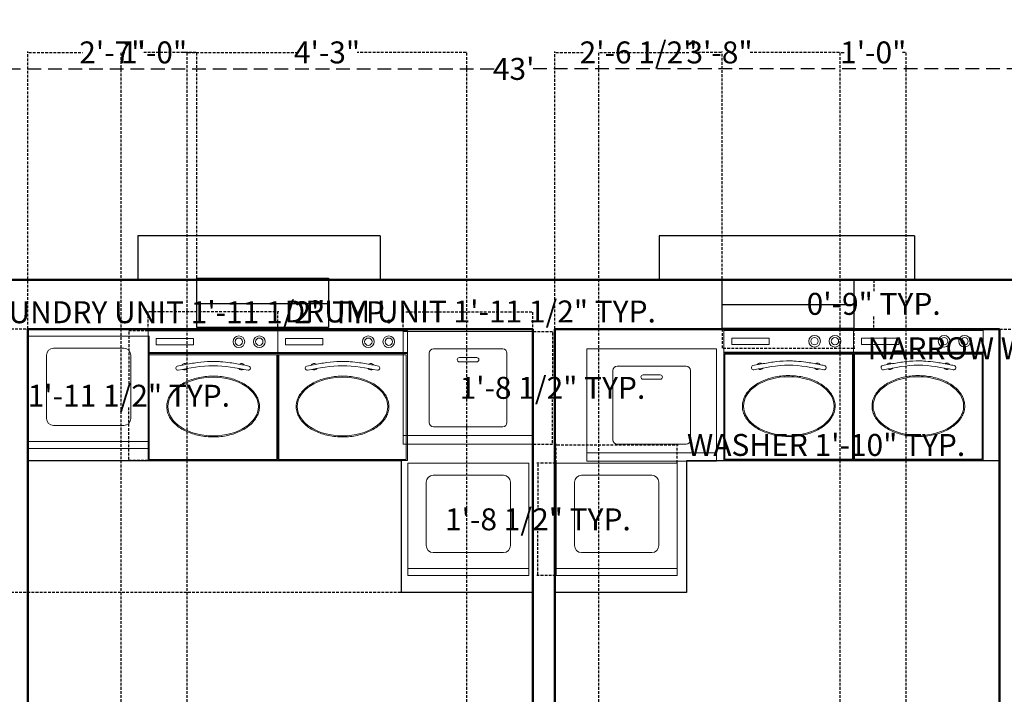
# Model space of a CAD drawing. Units: inches. Extents: x 513 to 1142, y 396 to 927.
# Tile 25 of 31: x 743 to 922, y 804 to 927. Entities that reach past the tile are written whole.
import ezdxf

# ---------------------------------------------------------------- set-up
doc = ezdxf.new("R2010")
doc.units = ezdxf.units.IN
doc.header["$MEASUREMENT"] = 0
doc.linetypes.add('DASHED', pattern=[0.75, 0.5, -0.25])
for name, color, linetype, lineweight in [('A-ANNO-DIMS', 2, 'DASHED', 18), ('A-EQPM', 92, 'Continuous', 18), ('A-FLOR-CASE', 7, 'Continuous', 25), ('A-WALL', 7, 'Continuous', 50), ('windows', 172, 'Continuous', 25)]:
    doc.layers.add(name, color=color, linetype=linetype, lineweight=lineweight)
doc.styles.get("Standard").update_dxf_attribs({"font": 'arial.ttf'})
doc.dimstyles.get("Standard").update_dxf_attribs({"dimtxt": 4, "dimasz": 0.18, "dimexe": 0.18, "dimexo": 0.0625, "dimgap": 0.09, "dimtad": 0, "dimtih": 1, "dimtoh": 1, "dimdec": 0, "dimrnd": 6, "dimzin": 0, "dimdsep": 46, "dimlunit": 3, "dimtxsty": 'Standard', "dimcen": 0.09, "dimadec": 0, "dimazin": 0, "dimtfac": 1, "dimtdec": 0, "dimtofl": 0, "dimtmove": 0, "dimatfit": 3, "dimfxl": 1, "dimtolj": 1, "dimtzin": 0, "dimarcsym": 0})

# ---------------------------------------------------------------- blocks, each defined once
blk = doc.blocks.new('A$C7E884C79')
for p, q in [((0, 0), (0, 600)), ((0, 600), (0, 0)), ((0, 600), (600, 600)), ((600, 600), (600, 0)), ((600, 0), (600, 600)), ((600, 600), (600, 450)), ((600, 600), (600, 500)), ((600, 500), (0, 500)), ((600, 495), (0, 495)), ((600, 500), (600, 0)), ((0, 0), (600, 0))]:
    blk.add_line(p, q)
for points in [[(36.4, 564.7), (208.9, 564.7), (208.9, 535.3), (36.4, 535.3)], [(5, 490), (595, 490), (595, 5), (5, 5)]]:
    blk.add_lwpolyline(points, close=True)
for centre, radius in [((419.3, 550), 27), ((419.3, 550), 17), ((513.9, 550), 27), ((513.9, 550), 17)]:
    blk.add_circle(centre, radius)
for centre, radius, start, end in [((137.2, 428), 10, 107.9829, 276.9581), ((168.5, 434.2), 15, 50.7888, 150.367), ((168.5, 434.2), 15, 234.0165, 327.1412), ((431.5, 434.2), 15, 212.8588, 305.9835), ((431.5, 434.2), 15, 29.633, 129.2112), ((462.8, 428), 10, 263.0419, 72.0171)]:
    blk.add_arc(centre, radius, start, end)
blk.add_ellipse((300, 250), major_axis=(-209.5, 0), ratio=0.648352)
for points, knots in [([(134.1, 437.5), (144.6, 439.5), (155.1, 441.6), (186, 447.3), (206.5, 450.9), (247.9, 456.4), (268.7, 458.3), (293.5, 458.9), (297.3, 458.9), (304.8, 458.9), (308.5, 458.8), (319.7, 458.5), (327.1, 458.1), (349.4, 456.5), (364.1, 454.9), (399.8, 449.9), (420.6, 446.2), (449.5, 440.7), (457.7, 439.1), (465.9, 437.5)], [0, 0, 0, 0, 31.638865, 31.638865, 92.600143, 92.600143, 153.561421, 153.561421, 164.367647, 164.367647, 175.173874, 175.173874, 196.786327, 196.786327, 240.011233, 240.011233, 302.099201, 302.099201, 326.773065, 326.773065, 326.773065, 326.773065]), ([(85.5, 250), (85.5, 244.8), (85.9, 239.6), (88, 226.9), (90.2, 219.4), (96.4, 204.8), (100.4, 197.7), (109.9, 184.1), (115.6, 177.5), (128.3, 165.1), (135.4, 159.2), (150.9, 148.3), (159.3, 143.3), (177.1, 134.2), (186.6, 130.1), (206.5, 123), (216.8, 119.9), (238.1, 114.9), (249, 113), (271.2, 110.2), (282.5, 109.4), (305, 109), (316.4, 109.4), (338.8, 111.3), (349.8, 112.8), (371.5, 117), (382.1, 119.6), (402.5, 126), (412.3, 129.7), (431, 138.1), (439.8, 142.8), (456.2, 153), (463.8, 158.6), (477.6, 170.5), (483.8, 176.8), (494.6, 190.1), (499.2, 197), (506.7, 211.3), (509.5, 218.7), (513.4, 233.6), (514.4, 241.3), (514.6, 256.5), (513.8, 264.1), (510.2, 279.1), (507.6, 286.6), (500.4, 300.9), (496, 307.9), (485.5, 321.3), (479.5, 327.7), (466, 339.7), (458.5, 345.3), (442.4, 355.8), (433.6, 360.5), (415.2, 369.1), (405.5, 373), (385.2, 379.5), (374.7, 382.3), (353.1, 386.7), (342, 388.3), (319.7, 390.5), (308.4, 390.9), (285.8, 390.7), (274.5, 390.1), (252.3, 387.5), (241.3, 385.7), (219.9, 380.9), (209.5, 378), (189.5, 371), (179.9, 367.1), (161.8, 358.1), (153.3, 353.2), (137.6, 342.5), (130.3, 336.7), (117.3, 324.4), (111.6, 317.9), (101.6, 304.3), (97.5, 297.3), (91, 282.8), (88.6, 275.3), (86, 261.9), (85.5, 255.9), (85.5, 250)], [0, 0, 0, 0, 0.108301, 0.108301, 0.267534, 0.267534, 0.426768, 0.426768, 0.586002, 0.586002, 0.745235, 0.745235, 0.904469, 0.904469, 1.063703, 1.063703, 1.222936, 1.222936, 1.38217, 1.38217, 1.541404, 1.541404, 1.700637, 1.700637, 1.859871, 1.859871, 2.019105, 2.019105, 2.178339, 2.178339, 2.337572, 2.337572, 2.496806, 2.496806, 2.65604, 2.65604, 2.815273, 2.815273, 2.974507, 2.974507, 3.133741, 3.133741, 3.292974, 3.292974, 3.452208, 3.452208, 3.611442, 3.611442, 3.770676, 3.770676, 3.929909, 3.929909, 4.089143, 4.089143, 4.248377, 4.248377, 4.40761, 4.40761, 4.566844, 4.566844, 4.726078, 4.726078, 4.885311, 4.885311, 5.044545, 5.044545, 5.203779, 5.203779, 5.363012, 5.363012, 5.522246, 5.522246, 5.68148, 5.68148, 5.840714, 5.840714, 5.999947, 5.999947, 6.159181, 6.159181, 6.283185, 6.283185, 6.283185, 6.283185])]:
    blk.add_open_spline(points, degree=3, knots=knots)
blk.add_open_spline([(138, 417.8), (192, 428.4), (300, 449.4), (408, 428.4), (462, 417.8)], degree=3)
blk = doc.blocks.new('LAVAD-01')
for p, q in [((-0.3221, 0.3585), (-0.3221, -0.3915)), ((0.3279, 0.3585), (-0.3221, 0.3585)), ((-0.2721, 0.3585), (-0.2721, -0.3915)), ((0.3279, -0.3915), (0.3279, 0.3585)), ((-0.2221, 0.1835), (-0.2221, -0.2165)), ((0.2029, 0.2085), (-0.1971, 0.2085)), ((0.2279, -0.2165), (0.2279, 0.1835)), ((0.1529, 0.0335), (0.1529, -0.0665)), ((0.1654, 0.046), (0.1654, 0.046)), ((0.1779, -0.0665), (0.1779, 0.0335)), ((0.1654, -0.079), (0.1654, -0.079)), ((-0.1971, -0.2415), (0.2029, -0.2415)), ((-0.3221, -0.3915), (0.3279, -0.3915))]:
    blk.add_line(p, q)
for centre, radius, start, end in [((-0.1971, 0.1835), 0.025, 90, 180), ((0.2029, 0.1835), 0.025, 0, 90), ((0.1654, 0.0335), 0.0125, 90, 180), ((0.1654, 0.0335), 0.0125, 0, 90), ((0.1654, -0.0665), 0.0125, 180, 270), ((0.1654, -0.0665), 0.0125, 270, 360), ((-0.1971, -0.2165), 0.025, 180, 270), ((0.2029, -0.2165), 0.025, 270, 360)]:
    blk.add_arc(centre, radius, start, end)
blk = doc.blocks.new('LAVADORA')
for p, q in [((-0.35, 0.65), (-0.35, 0)), ((-0.35, 0.65), (0.35, 0.65)), ((0.35, 0.65), (0.35, 0)), ((-0.2031, 0.5795), (0.2031, 0.5795)), ((-0.2437, 0.5389), (-0.2437, 0.1732)), ((0.2437, 0.5389), (0.2437, 0.1732)), ((-0.2031, 0.1326), (0.2031, 0.1326)), ((-0.35, 0.0406), (0.35, 0.0406)), ((-0.35, 0), (0.35, 0))]:
    blk.add_line(p, q)
for centre, start, end in [((-0.2031, 0.5389), 90, 180), ((0.2031, 0.5389), 0, 90), ((-0.2031, 0.1732), 180, 270), ((0.2031, 0.1732), 270, 0)]:
    blk.add_arc(centre, 0.0406, start, end)
blk = doc.blocks.new('*D103')
at = {"layer": 'A-ANNO-DIMS', "color": 0, "lineweight": -2, "ltscale": 5, "transparency": 16777216}
for p, q in [((575, 879.22), (575, 917.74)), ((575.18, 917.56), (828.93, 917.56)), ((1089.82, 917.56), (836.06, 917.56)), ((1090, 879.22), (1090, 917.74))]:
    blk.add_line(p, q, dxfattribs=at)
at = {"layer": 'A-ANNO-DIMS', "color": 0, "ltscale": 5, "transparency": 16777216}
for points in [[(575.18, 917.59), (575.18, 917.53), (575, 917.56)], [(1089.82, 917.59), (1089.82, 917.53), (1090, 917.56)]]:
    blk.add_solid(points, dxfattribs=at)
at = {"layer": 'Defpoints', "color": 0, "ltscale": 5, "transparency": 16777216}
for p in [(1090, 917.56), (575, 879.16), (1090, 879.16)]:
    blk.add_point(p, dxfattribs=at)
at = {"layer": 'A-ANNO-DIMS', "color": 0, "ltscale": 5, "transparency": 16777216, "insert": (832.5, 917.56), "char_height": 4, "attachment_point": 5}
blk.add_mtext("\\A1;43'", dxfattribs=at)
blk = doc.blocks.new('WIN-24IN')
blk.add_line((0, 4.39), (24, 4.39))
blk.add_lwpolyline([(24, 0), (0, 0), (0, 9), (24, 9)], close=True)
blk = doc.blocks.new('*D111')
at = {"layer": 'A-ANNO-DIMS', "color": 0, "lineweight": -2, "transparency": 16777216}
for p, q in [((765.94, 869.89), (765.94, 873.55)), ((789.56, 869.89), (789.56, 873.55)), ((766.12, 873.37), (789.38, 873.37)), ((789.56, 873.37), (789.74, 873.37))]:
    blk.add_line(p, q, dxfattribs=at)
at = {"layer": 'A-ANNO-DIMS', "color": 0, "transparency": 16777216}
for points in [[(766.12, 873.4), (766.12, 873.34), (765.94, 873.37)], [(789.38, 873.4), (789.38, 873.34), (789.56, 873.37)]]:
    blk.add_solid(points, dxfattribs=at)
at = {"layer": 'Defpoints', "color": 0, "transparency": 16777216}
for p in [(789.56, 873.37), (765.94, 869.83), (789.56, 869.83)]:
    blk.add_point(p, dxfattribs=at)
at = {"layer": 'A-ANNO-DIMS', "color": 0, "transparency": 16777216, "insert": (824.59, 873.37), "char_height": 4, "attachment_point": 5}
blk.add_mtext('\\A1;DRUM UNIT 1\'-11 1/2" TYP.', dxfattribs=at)
blk = doc.blocks.new('*D112')
at = {"layer": 'A-ANNO-DIMS', "color": 0, "lineweight": -2, "transparency": 16777216}
for p, q in [((765.88, 869.83), (762.22, 869.83)), ((762.4, 869.65), (762.4, 860.18)), ((762.4, 846.39), (762.4, 855.86)), ((765.88, 846.21), (762.22, 846.21))]:
    blk.add_line(p, q, dxfattribs=at)
at = {"layer": 'A-ANNO-DIMS', "color": 0, "transparency": 16777216}
for points in [[(762.37, 869.65), (762.43, 869.65), (762.4, 869.83)], [(762.37, 846.39), (762.43, 846.39), (762.4, 846.21)]]:
    blk.add_solid(points, dxfattribs=at)
at = {"layer": 'Defpoints', "color": 0, "transparency": 16777216}
for p in [(762.4, 869.83), (765.94, 869.83), (765.94, 846.21)]:
    blk.add_point(p, dxfattribs=at)
at = {"layer": 'A-ANNO-DIMS', "color": 0, "transparency": 16777216, "insert": (762.4, 858.02), "char_height": 4, "attachment_point": 5}
blk.add_mtext('\\A1;1\'-11 1/2" TYP.', dxfattribs=at)
blk = doc.blocks.new('*D113')
at = {"layer": 'A-ANNO-DIMS', "color": 0, "lineweight": -2, "transparency": 16777216}
for p, q in [((840.22, 845.81), (840.22, 849.24)), ((840.4, 849.06), (862.09, 849.06)), ((862.27, 845.81), (862.27, 849.24)), ((862.27, 849.06), (862.45, 849.06))]:
    blk.add_line(p, q, dxfattribs=at)
at = {"layer": 'A-ANNO-DIMS', "color": 0, "transparency": 16777216}
for points in [[(840.4, 849.09), (840.4, 849.03), (840.22, 849.06)], [(862.09, 849.09), (862.09, 849.03), (862.27, 849.06)]]:
    blk.add_solid(points, dxfattribs=at)
at = {"layer": 'Defpoints', "color": 0, "transparency": 16777216}
for p in [(862.27, 849.06), (840.22, 845.75), (862.27, 845.75)]:
    blk.add_point(p, dxfattribs=at)
at = {"layer": 'A-ANNO-DIMS', "color": 0, "transparency": 16777216, "insert": (889.41, 849.06), "char_height": 4, "attachment_point": 5}
blk.add_mtext('\\A1;WASHER 1\'-10" TYP.', dxfattribs=at)
blk = doc.blocks.new('*D114')
at = {"layer": 'A-ANNO-DIMS', "color": 0, "lineweight": -2, "transparency": 16777216}
for p, q in [((840.16, 845.75), (836.74, 845.75)), ((836.92, 845.57), (836.92, 837.67)), ((836.92, 825.46), (836.92, 833.35)), ((840.16, 825.28), (836.74, 825.28))]:
    blk.add_line(p, q, dxfattribs=at)
at = {"layer": 'A-ANNO-DIMS', "color": 0, "transparency": 16777216}
for points in [[(836.89, 845.57), (836.95, 845.57), (836.92, 845.75)], [(836.89, 825.46), (836.95, 825.46), (836.92, 825.28)]]:
    blk.add_solid(points, dxfattribs=at)
at = {"layer": 'Defpoints', "color": 0, "transparency": 16777216}
for p in [(836.92, 845.75), (840.22, 845.75), (840.22, 825.28)]:
    blk.add_point(p, dxfattribs=at)
at = {"layer": 'A-ANNO-DIMS', "color": 0, "transparency": 16777216, "insert": (836.92, 835.51), "char_height": 4, "attachment_point": 5}
blk.add_mtext('\\A1;1\'-8 1/2" TYP.', dxfattribs=at)
blk = doc.blocks.new('*D115')
at = {"layer": 'A-ANNO-DIMS', "color": 0, "lineweight": -2, "transparency": 16777216}
for p, q in [((812.39, 873.24), (812.21, 873.24)), ((812.39, 869.76), (812.39, 873.42)), ((835.83, 873.24), (812.57, 873.24)), ((836.01, 869.76), (836.01, 873.42))]:
    blk.add_line(p, q, dxfattribs=at)
at = {"layer": 'A-ANNO-DIMS', "color": 0, "transparency": 16777216}
for points in [[(812.57, 873.27), (812.57, 873.21), (812.39, 873.24)], [(835.83, 873.27), (835.83, 873.21), (836.01, 873.24)]]:
    blk.add_solid(points, dxfattribs=at)
at = {"layer": 'Defpoints', "color": 0, "transparency": 16777216}
for p in [(812.39, 873.24), (812.39, 869.7), (836.01, 869.7)]:
    blk.add_point(p, dxfattribs=at)
at = {"layer": 'A-ANNO-DIMS', "color": 0, "transparency": 16777216, "insert": (772.38, 873.24), "char_height": 4, "attachment_point": 5}
blk.add_mtext('\\A1;LAUNDRY UNIT 1\'-11 1/2" TYP.', dxfattribs=at)
blk = doc.blocks.new('*D116')
at = {"layer": 'A-ANNO-DIMS', "color": 0, "lineweight": -2, "transparency": 16777216}
for p, q in [((836.08, 869.7), (839.74, 869.7)), ((839.56, 869.52), (839.56, 861.62)), ((839.56, 849.41), (839.56, 857.31)), ((836.08, 849.23), (839.74, 849.23))]:
    blk.add_line(p, q, dxfattribs=at)
at = {"layer": 'A-ANNO-DIMS', "color": 0, "transparency": 16777216}
for points in [[(839.53, 869.52), (839.59, 869.52), (839.56, 869.7)], [(839.53, 849.41), (839.59, 849.41), (839.56, 849.23)]]:
    blk.add_solid(points, dxfattribs=at)
at = {"layer": 'Defpoints', "color": 0, "transparency": 16777216}
for p in [(836.01, 869.7), (839.56, 869.7), (836.01, 849.23)]:
    blk.add_point(p, dxfattribs=at)
at = {"layer": 'A-ANNO-DIMS', "color": 0, "transparency": 16777216, "insert": (839.56, 859.46), "char_height": 4, "attachment_point": 5}
blk.add_mtext('\\A1;1\'-8 1/2" TYP.', dxfattribs=at)
blk = doc.blocks.new('*D129')
at = {"layer": 'A-ANNO-DIMS', "color": 0, "lineweight": -2, "transparency": 16777216}
for p, q in [((870.48, 870.2), (870.48, 866.48)), ((894.48, 870.2), (894.48, 866.48)), ((870.66, 866.66), (894.3, 866.66)), ((894.48, 866.66), (894.66, 866.66))]:
    blk.add_line(p, q, dxfattribs=at)
at = {"layer": 'A-ANNO-DIMS', "color": 0, "transparency": 16777216}
for points in [[(870.66, 866.69), (870.66, 866.63), (870.48, 866.66)], [(894.3, 866.69), (894.3, 866.63), (894.48, 866.66)]]:
    blk.add_solid(points, dxfattribs=at)
at = {"layer": 'Defpoints', "color": 0, "transparency": 16777216}
for p in [(870.48, 870.26), (894.48, 870.26), (894.48, 866.66)]:
    blk.add_point(p, dxfattribs=at)
at = {"layer": 'A-ANNO-DIMS', "color": 0, "transparency": 16777216, "insert": (933.38, 866.66), "char_height": 4, "attachment_point": 5}
blk.add_mtext('\\A1;NARROW WINDOW 2\'-0" TYP.', dxfattribs=at)
blk = doc.blocks.new('*D130')
at = {"layer": 'A-ANNO-DIMS', "color": 0, "lineweight": -2, "transparency": 16777216}
for p, q in [((894.54, 879.26), (898.26, 879.26)), ((898.08, 879.08), (898.08, 876.9)), ((898.08, 870.44), (898.08, 872.63)), ((894.54, 870.26), (898.26, 870.26))]:
    blk.add_line(p, q, dxfattribs=at)
at = {"layer": 'A-ANNO-DIMS', "color": 0, "transparency": 16777216}
for points in [[(898.05, 879.08), (898.11, 879.08), (898.08, 879.26)], [(898.05, 870.44), (898.11, 870.44), (898.08, 870.26)]]:
    blk.add_solid(points, dxfattribs=at)
at = {"layer": 'Defpoints', "color": 0, "transparency": 16777216}
for p in [(894.48, 879.26), (898.08, 879.26), (894.48, 870.26)]:
    blk.add_point(p, dxfattribs=at)
at = {"layer": 'A-ANNO-DIMS', "color": 0, "transparency": 16777216, "insert": (898.08, 874.76), "char_height": 4, "attachment_point": 5}
blk.add_mtext('\\A1;0\'-9" TYP.', dxfattribs=at)
blk = doc.blocks.new('*D148')
at = {"layer": 'A-ANNO-DIMS', "color": 0, "lineweight": -2, "transparency": 16777216}
for p, q in [((921.06, 870.16), (1131.58, 870.16)), ((1131.4, 869.98), (1131.4, 824.29)), ((1131.4, 774.34), (1131.4, 820.03)), ((897.06, 774.16), (1131.58, 774.16))]:
    blk.add_line(p, q, dxfattribs=at)
at = {"layer": 'A-ANNO-DIMS', "color": 0, "transparency": 16777216}
for points in [[(1131.37, 869.98), (1131.43, 869.98), (1131.4, 870.16)], [(1131.37, 774.34), (1131.43, 774.34), (1131.4, 774.16)]]:
    blk.add_solid(points, dxfattribs=at)
at = {"layer": 'Defpoints', "color": 0, "transparency": 16777216}
for p in [(921, 870.16), (1131.4, 870.16), (897, 774.16)]:
    blk.add_point(p, dxfattribs=at)
at = {"layer": 'A-ANNO-DIMS', "color": 0, "transparency": 16777216, "insert": (1131.4, 822.16), "char_height": 4, "attachment_point": 5}
blk.add_mtext('\\A1;8\'-0"', dxfattribs=at)
blk = doc.blocks.new('*D153')
at = {"layer": 'A-ANNO-DIMS', "color": 0, "lineweight": -2, "transparency": 16777216}
for p, q in [((744, 870.22), (744, 920.74)), ((744.18, 920.56), (753.95, 920.56)), ((774.61, 920.56), (764.83, 920.56)), ((774.79, 870.5), (774.79, 920.74))]:
    blk.add_line(p, q, dxfattribs=at)
at = {"layer": 'A-ANNO-DIMS', "color": 0, "transparency": 16777216}
for points in [[(744.18, 920.59), (744.18, 920.53), (744, 920.56)], [(774.61, 920.59), (774.61, 920.53), (774.79, 920.56)]]:
    blk.add_solid(points, dxfattribs=at)
at = {"layer": 'Defpoints', "color": 0, "transparency": 16777216}
for p in [(774.79, 920.56), (744, 870.16), (774.79, 870.44)]:
    blk.add_point(p, dxfattribs=at)
at = {"layer": 'A-ANNO-DIMS', "color": 0, "transparency": 16777216, "insert": (759.39, 920.56), "char_height": 4, "attachment_point": 5}
blk.add_mtext('\\A1;2\'-7"', dxfattribs=at)
blk = doc.blocks.new('*D154')
at = {"layer": 'A-ANNO-DIMS', "color": 0, "lineweight": -2, "transparency": 16777216}
for p, q in [((840, 870.22), (840, 920.74)), ((840.18, 920.56), (845.14, 920.56)), ((870.3, 920.56), (865.34, 920.56)), ((870.48, 870.33), (870.48, 920.74))]:
    blk.add_line(p, q, dxfattribs=at)
at = {"layer": 'A-ANNO-DIMS', "color": 0, "transparency": 16777216}
for points in [[(840.18, 920.59), (840.18, 920.53), (840, 920.56)], [(870.3, 920.59), (870.3, 920.53), (870.48, 920.56)]]:
    blk.add_solid(points, dxfattribs=at)
at = {"layer": 'Defpoints', "color": 0, "transparency": 16777216}
for p in [(870.48, 920.56), (840, 870.16), (870.48, 870.26)]:
    blk.add_point(p, dxfattribs=at)
at = {"layer": 'A-ANNO-DIMS', "color": 0, "transparency": 16777216, "insert": (855.24, 920.56), "char_height": 4, "attachment_point": 5}
blk.add_mtext('\\A1;2\'-6 1/2"', dxfattribs=at)
blk = doc.blocks.new('*D167')
at = {"layer": 'A-ANNO-DIMS', "color": 0, "lineweight": -2, "transparency": 16777216}
for p, q in [((761, 637.22), (761, 920.74)), ((761.18, 920.56), (761.78, 920.56)), ((772.82, 920.56), (772.21, 920.56)), ((773, 637.22), (773, 920.74))]:
    blk.add_line(p, q, dxfattribs=at)
at = {"layer": 'A-ANNO-DIMS', "color": 0, "transparency": 16777216}
for points in [[(761.18, 920.59), (761.18, 920.53), (761, 920.56)], [(772.82, 920.59), (772.82, 920.53), (773, 920.56)]]:
    blk.add_solid(points, dxfattribs=at)
at = {"layer": 'Defpoints', "color": 0, "transparency": 16777216}
for p in [(773, 920.56), (761, 637.16), (773, 637.16)]:
    blk.add_point(p, dxfattribs=at)
at = {"layer": 'A-ANNO-DIMS', "color": 0, "transparency": 16777216, "insert": (767, 920.56), "char_height": 4, "attachment_point": 5}
blk.add_mtext('\\A1;1\'-0"', dxfattribs=at)
blk = doc.blocks.new('*D168')
at = {"layer": 'A-ANNO-DIMS', "color": 0, "lineweight": -2, "transparency": 16777216}
for p, q in [((892, 637.22), (892, 920.74)), ((892.18, 920.56), (892.78, 920.56)), ((903.82, 920.56), (903.21, 920.56)), ((904, 637.22), (904, 920.74))]:
    blk.add_line(p, q, dxfattribs=at)
at = {"layer": 'A-ANNO-DIMS', "color": 0, "transparency": 16777216}
for points in [[(892.18, 920.59), (892.18, 920.53), (892, 920.56)], [(903.82, 920.59), (903.82, 920.53), (904, 920.56)]]:
    blk.add_solid(points, dxfattribs=at)
at = {"layer": 'Defpoints', "color": 0, "transparency": 16777216}
for p in [(904, 920.56), (892, 637.16), (904, 637.16)]:
    blk.add_point(p, dxfattribs=at)
at = {"layer": 'A-ANNO-DIMS', "color": 0, "transparency": 16777216, "insert": (898, 920.56), "char_height": 4, "attachment_point": 5}
blk.add_mtext('\\A1;1\'-0"', dxfattribs=at)
blk = doc.blocks.new('*D170')
at = {"layer": 'A-ANNO-DIMS', "color": 0, "lineweight": -2, "transparency": 16777216}
for p, q in [((835.93, 870.16), (533.42, 870.16)), ((533.6, 869.98), (533.6, 848.29)), ((533.6, 822.34), (533.6, 844.03)), ((835.93, 822.16), (533.42, 822.16))]:
    blk.add_line(p, q, dxfattribs=at)
at = {"layer": 'A-ANNO-DIMS', "color": 0, "transparency": 16777216}
for points in [[(533.57, 869.98), (533.63, 869.98), (533.6, 870.16)], [(533.57, 822.34), (533.63, 822.34), (533.6, 822.16)]]:
    blk.add_solid(points, dxfattribs=at)
at = {"layer": 'Defpoints', "color": 0, "transparency": 16777216}
for p in [(533.6, 870.16), (836, 870.16), (836, 822.16)]:
    blk.add_point(p, dxfattribs=at)
at = {"layer": 'A-ANNO-DIMS', "color": 0, "transparency": 16777216, "insert": (533.6, 846.16), "char_height": 4, "attachment_point": 5}
blk.add_mtext('\\A1;4\'-0"', dxfattribs=at)
blk = doc.blocks.new('*D175')
at = {"layer": 'A-ANNO-DIMS', "color": 0, "lineweight": -2, "transparency": 16777216}
for p, q in [((773, 637.22), (773, 920.74)), ((773.18, 920.56), (793.01, 920.56)), ((823.82, 920.56), (803.98, 920.56)), ((824, 637.22), (824, 920.74))]:
    blk.add_line(p, q, dxfattribs=at)
at = {"layer": 'A-ANNO-DIMS', "color": 0, "transparency": 16777216}
for points in [[(773.18, 920.59), (773.18, 920.53), (773, 920.56)], [(823.82, 920.59), (823.82, 920.53), (824, 920.56)]]:
    blk.add_solid(points, dxfattribs=at)
at = {"layer": 'Defpoints', "color": 0, "transparency": 16777216}
for p in [(824, 920.56), (773, 637.16), (824, 637.16)]:
    blk.add_point(p, dxfattribs=at)
at = {"layer": 'A-ANNO-DIMS', "color": 0, "transparency": 16777216, "insert": (798.5, 920.56), "char_height": 4, "attachment_point": 5}
blk.add_mtext('\\A1;4\'-3"', dxfattribs=at)
blk = doc.blocks.new('*D176')
at = {"layer": 'A-ANNO-DIMS', "color": 0, "lineweight": -2, "transparency": 16777216}
for p, q in [((848, 637.22), (848, 920.74)), ((848.18, 920.56), (864.59, 920.56)), ((891.82, 920.56), (875.4, 920.56)), ((892, 637.22), (892, 920.74))]:
    blk.add_line(p, q, dxfattribs=at)
at = {"layer": 'A-ANNO-DIMS', "color": 0, "transparency": 16777216}
for points in [[(848.18, 920.59), (848.18, 920.53), (848, 920.56)], [(891.82, 920.59), (891.82, 920.53), (892, 920.56)]]:
    blk.add_solid(points, dxfattribs=at)
at = {"layer": 'Defpoints', "color": 0, "transparency": 16777216}
for p in [(892, 920.56), (848, 637.16), (892, 637.16)]:
    blk.add_point(p, dxfattribs=at)
at = {"layer": 'A-ANNO-DIMS', "color": 0, "transparency": 16777216, "insert": (870, 920.56), "char_height": 4, "attachment_point": 5}
blk.add_mtext('\\A1;3\'-8"', dxfattribs=at)

msp = doc.modelspace()

# ---------------------------------------------------------------- linework, layer by layer
at = {"layer": 'A-FLOR-CASE'}
for p, q in [((812, 846.16), (744, 846.16)), ((812, 846.16), (812, 822.16)), ((921, 846.16), (864, 846.16)), ((864, 846.16), (864, 822.16)), ((836, 822.16), (812, 822.16)), ((864, 822.16), (840, 822.16))]:
    msp.add_line(p, q, dxfattribs=at)
at = {"layer": 'A-WALL'}
for p, q in [((1090, 879.16), (575, 879.16)), ((744, 870.16), (744, 710.16)), ((836, 870.16), (744, 870.16)), ((836, 870.16), (836, 774.16)), ((840, 870.16), (840, 774.16)), ((921, 870.16), (840, 870.16)), ((921, 710.16), (921, 870.16))]:
    msp.add_line(p, q, dxfattribs=at)
at = {"layer": 'windows'}
for p, q in [((764.02, 887.16), (764.02, 879.16)), ((808.21, 887.16), (764.02, 887.16)), ((808.21, 887.16), (808.21, 879.16)), ((859.02, 887.16), (859.02, 879.16)), ((905.5, 887.16), (859.02, 887.16)), ((905.5, 887.16), (905.5, 879.16))]:
    msp.add_line(p, q, dxfattribs=at)

# ---------------------------------------------------------------- block references
at = {"layer": 'A-EQPM'}
for name, p, xscale, yscale, zscale in [('A$C7E884C79', (870.8, 846.3), 0.0393700787401575, 0.0393700787401575, 0.0393700787401575), ('A$C7E884C79', (894.41, 846.3), 0.0393700787401575, 0.0393700787401575, 0.0393700787401575), ('LAVADORA', (755.08, 848.43), 31.49606299212599, 31.49606299212599, 31.49606299212599), ('A$C7E884C79', (765.94, 846.21), 0.0393700787401575, 0.0393700787401575, 0.0393700787401575), ('A$C7E884C79', (789.52, 846.21), 0.0393700787401575, 0.0393700787401575, 0.0393700787401575), ('LAVADORA', (824.25, 825.28), 31.49606299212599, 31.49606299212599, 31.49606299212599), ('LAVADORA', (851.25, 825.28), 31.49606299212599, 31.49606299212599, 31.49606299212599)]:
    msp.add_blockref(name, p, dxfattribs=dict(at, xscale=xscale, yscale=yscale, zscale=zscale))
at = {"layer": 'A-EQPM', "xscale": 31.49606299212599, "yscale": 31.49606299212599, "zscale": 31.49606299212599, "rotation": 90}
for p in [(823.68, 859.37), (857.12, 856.22)]:
    msp.add_blockref('LAVAD-01', p, dxfattribs=at)
at = {"layer": 'windows'}
for p in [(774.79, 870.44), (870.48, 870.26)]:
    msp.add_blockref('WIN-24IN', p, dxfattribs=at)

# ---------------------------------------------------------------- dimensions: what is measured, and where the dimension line sits
at = {"layer": 'A-ANNO-DIMS'}
for base, p1, p2, picture, middle in [((870.48, 920.56), (840, 870.16), (870.48, 870.26), '*D154', (855.24, 920.56)), ((774.79, 920.56), (744, 870.16), (774.79, 870.44), '*D153', (759.39, 920.56)), ((773, 920.56), (761, 637.16), (773, 637.16), '*D167', (767, 920.56)), ((824, 920.56), (773, 637.16), (824, 637.16), '*D175', (798.5, 920.56)), ((892, 920.56), (848, 637.16), (892, 637.16), '*D176', (870, 920.56)), ((904, 920.56), (892, 637.16), (904, 637.16), '*D168', (898, 920.56))]:
    dim = msp.add_linear_dim(base=base, p1=p1, p2=p2, dimstyle='Standard', override={"dimdec": 1, "dimlfac": 1, "dimrnd": 0, "dimzin": 1, "dimdsep": 46, "dimlunit": 4, "dimfrac": 2}, dxfattribs=at)
    dim.commit()
    dim.dimension.update_dxf_attribs({"geometry": picture, "text_midpoint": middle})
at = {"layer": 'A-ANNO-DIMS', "ltscale": 5}
dim = msp.add_linear_dim(base=(1090, 917.56), p1=(575, 879.16), p2=(1090, 879.16), dimstyle='Standard', override={"dimclrd": 0, "dimclre": 0, "dimclrt": 0}, dxfattribs=at)
dim.commit()
dim.dimension.update_dxf_attribs({"geometry": '*D103', "text_midpoint": (832.5, 917.56)})
at = {"layer": 'A-ANNO-DIMS'}
for base, p1, p2, angle, text, picture, middle in [((812.39, 873.24), (836.01, 869.7), (812.39, 869.7), 180, 'LAUNDRY UNIT <> TYP.', '*D115', (772.38, 873.24)), ((898.08, 879.26), (894.48, 870.26), (894.48, 879.26), 90, '<> TYP.', '*D130', (898.08, 874.76)), ((762.4, 869.83), (765.94, 846.21), (765.94, 869.83), 90, '<> TYP.', '*D112', (762.4, 858.02)), ((839.56, 869.7), (836.01, 849.23), (836.01, 869.7), 90, '<> TYP.', '*D116', (839.56, 859.46)), ((836.92, 845.75), (840.22, 825.28), (840.22, 845.75), 90, '<> TYP.', '*D114', (836.92, 835.51))]:
    dim = msp.add_linear_dim(base=base, p1=p1, p2=p2, angle=angle, text=text, dimstyle='Standard', override={"dimdec": 1, "dimlfac": 1, "dimrnd": 0, "dimzin": 1, "dimdsep": 46, "dimlunit": 4, "dimfrac": 2}, dxfattribs=at)
    dim.commit()
    dim.dimension.update_dxf_attribs({"geometry": picture, "text_midpoint": middle})
for base, p1, p2, text, picture, middle in [((789.56, 873.37), (765.94, 869.83), (789.56, 869.83), 'DRUM UNIT <> TYP.', '*D111', (824.59, 873.37)), ((894.48, 866.66), (870.48, 870.26), (894.48, 870.26), 'NARROW WINDOW <> TYP.', '*D129', (933.38, 866.66)), ((862.2716, 849.055), (840.2243, 845.7479), (862.2716, 845.7479), 'WASHER <> TYP.', '*D113', (889.4079, 849.055))]:
    dim = msp.add_linear_dim(base=base, p1=p1, p2=p2, text=text, dimstyle='Standard', override={"dimdec": 1, "dimlfac": 1, "dimrnd": 0, "dimzin": 1, "dimdsep": 46, "dimlunit": 4, "dimfrac": 2}, dxfattribs=at)
    dim.commit()
    dim.dimension.update_dxf_attribs({"geometry": picture, "text_midpoint": middle})
for base, p1, p2, picture, middle in [((533.6, 870.16), (836, 822.16), (836, 870.16), '*D170', (533.6, 846.16)), ((1131.4, 870.16), (897, 774.16), (921, 870.16), '*D148', (1131.4, 822.16))]:
    dim = msp.add_linear_dim(base=base, p1=p1, p2=p2, angle=90, dimstyle='Standard', override={"dimdec": 1, "dimlfac": 1, "dimrnd": 0, "dimzin": 1, "dimdsep": 46, "dimlunit": 4, "dimfrac": 2}, dxfattribs=at)
    dim.commit()
    dim.dimension.update_dxf_attribs({"geometry": picture, "text_midpoint": middle})

doc.saveas('drawing.dxf')
